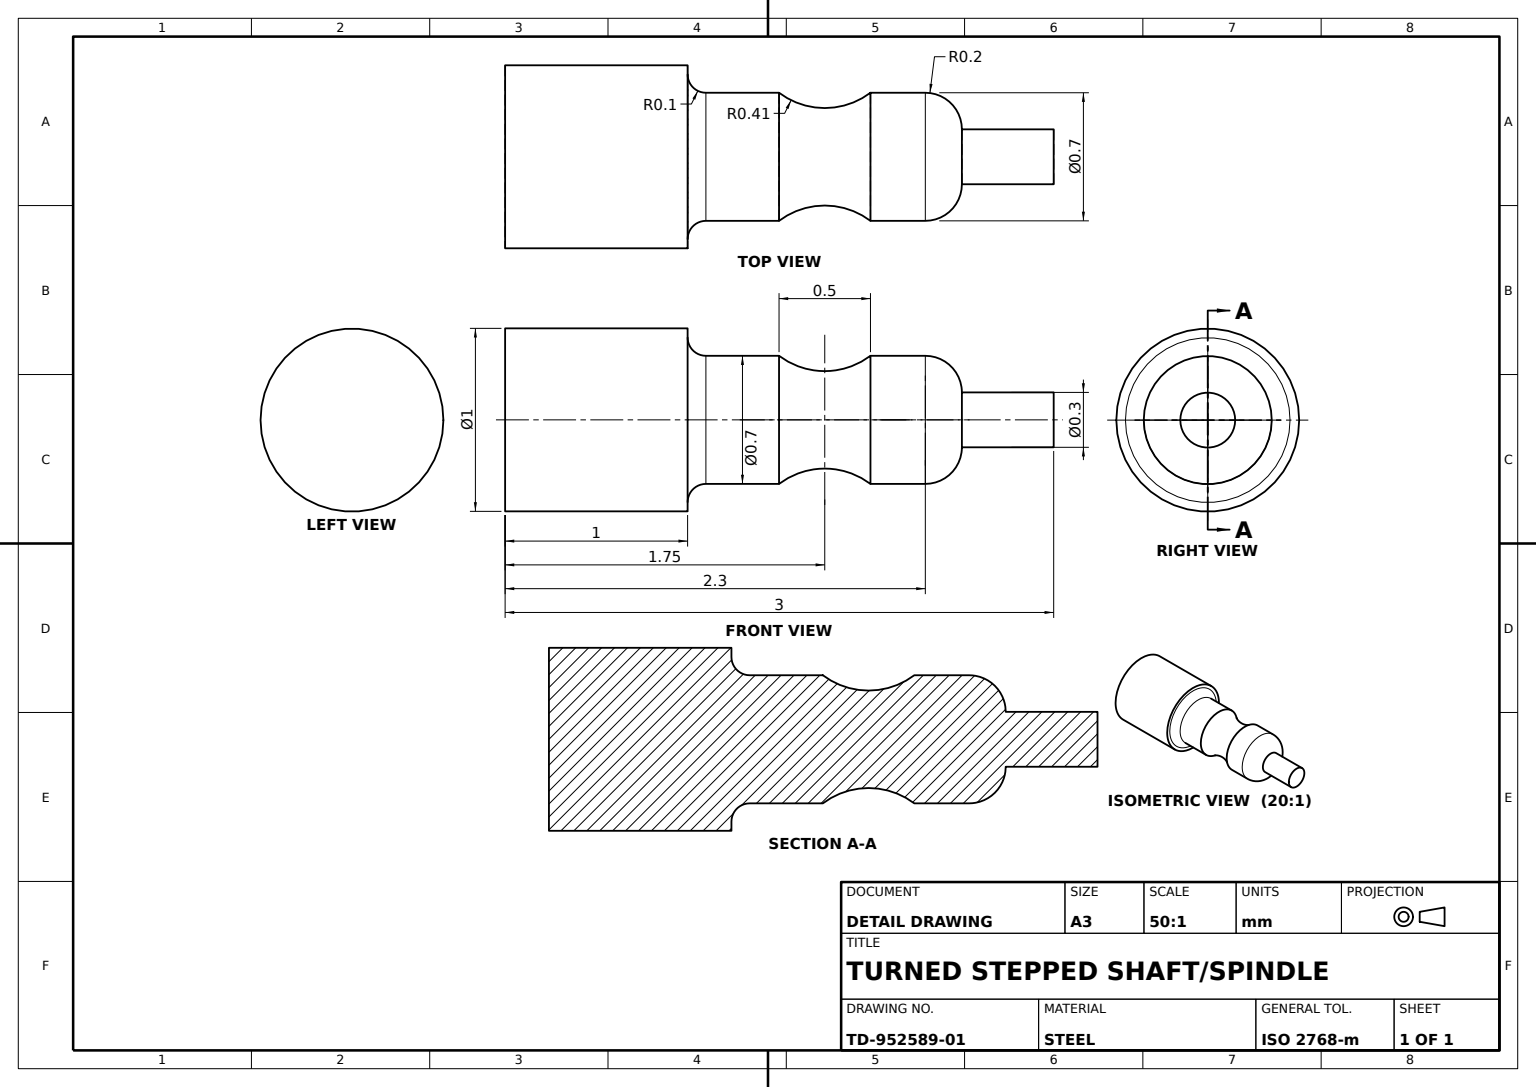
from build123d import *


with BuildPart() as part:
    # Pin Profile Sketch → Stepped Pin Revolve (revolve)
    with BuildSketch(Plane.XY, mode=Mode.PRIVATE) as stepped_pin_revolve_sk:
        with BuildLine():
            Line((3, 0), (3, -0.15))
            Line((3, -0.15), (2.498017858, -0.15))
            ThreePointArc((2.498017858, -0.15), (2.439439214, -0.291421356), (2.298017858, -0.35))
            Line((2.298017858, -0.35), (1.998017858, -0.35))
            ThreePointArc((1.998017858, -0.35), (1.748017858, -0.266247642), (1.498017858, -0.35))
            Line((1.498017858, -0.35), (1.098017858, -0.35))
            ThreePointArc((1.098017858, -0.35), (1.02730718, -0.379289322), (0.998017858, -0.45))
            Line((0.998017858, -0.45), (0.998017858, -0.5))
            Line((0.998017858, -0.5), (0, -0.5))
            Line((0, -0.5), (0, 0))
            Line((0, 0), (3, 0))
        make_face()
    revolve(stepped_pin_revolve_sk.sketch.rotate(Axis((0, 0, 0), (1, 0, 0)), 270), axis=Axis((0, 0, 0), (1, 0, 0)))


solid = part.part
